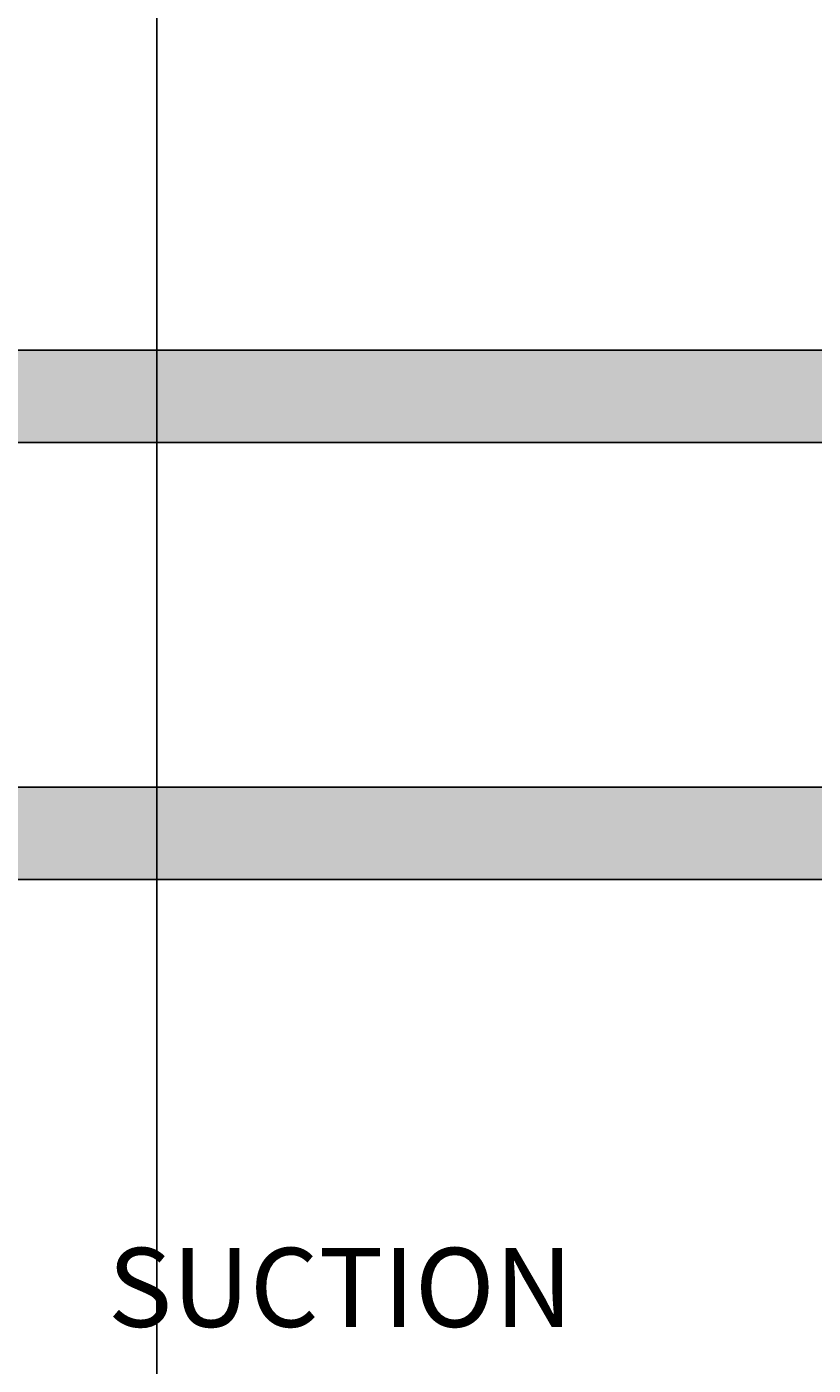
# Model space of a CAD drawing. Units: millimetres. Extents: x -11 to 280, y -4 to 208.
# Tile 5 of 55: x 61 to 91, y 36 to 87. Entities that reach past the tile are written whole.
import ezdxf

# ---------------------------------------------------------------- set-up
doc = ezdxf.new("R2010")
doc.units = ezdxf.units.MM
for name, color, linetype, lineweight in [('M-ANNO-TEXT', 7, 'Continuous', 18), ('M-DIMS', 2, 'Continuous', 18), ('M-HYDR-RETN', 7, 'Continuous', 25)]:
    doc.layers.add(name, color=color, linetype=linetype, lineweight=lineweight)
doc.layers.add('M-HYDR-RETN-PATT', color=114, linetype='Continuous', lineweight=13, true_color=0x139b48)
doc.styles.get("Standard").update_dxf_attribs({"font": 'arial.ttf'})
doc.dimstyles.get("Standard").update_dxf_attribs({"dimtxt": 0.18, "dimasz": 0.18, "dimexe": 0.18, "dimexo": 0.0625, "dimgap": 0.09, "dimtad": 0, "dimtih": 1, "dimtoh": 1, "dimdec": 4, "dimzin": 0, "dimdsep": 46, "dimtxsty": 'Standard', "dimcen": 0.09, "dimadec": 0, "dimazin": 0, "dimtfac": 1, "dimtdec": 4, "dimtofl": 0, "dimtmove": 0, "dimatfit": 3, "dimfxl": 1, "dimtolj": 1, "dimtzin": 0, "dimarcsym": 0})

# ---------------------------------------------------------------- blocks, each defined once
blk = doc.blocks.new('*D4')
at = {"layer": 'Defpoints', "color": 0, "transparency": 16777216}
for p in [(4.763, 84.426), (266.035, 51.733), (266.035, -3.415)]:
    blk.add_point(p, dxfattribs=at)
at = {"layer": 'M-DIMS', "color": 0, "lineweight": -2, "transparency": 16777216}
for p, q in [((4.763, 84.364), (4.763, -3.595)), ((266.035, 51.67), (266.035, -3.595)), ((4.943, -3.415), (134.934, -3.415)), ((265.855, -3.415), (135.864, -3.415))]:
    blk.add_line(p, q, dxfattribs=at)
at = {"layer": 'M-DIMS', "color": 0, "transparency": 16777216}
for points in [[(4.943, -3.385), (4.943, -3.445), (4.763, -3.415)], [(265.855, -3.385), (265.855, -3.445), (266.035, -3.415)]]:
    blk.add_solid(points, dxfattribs=at)
at = {"layer": 'M-DIMS', "color": 0, "transparency": 16777216, "insert": (135.399, -3.415), "char_height": 0.18, "attachment_point": 5}
blk.add_mtext('\\A1;261.27', dxfattribs=at)
blk = doc.blocks.new('*D5')
at = {"layer": 'Defpoints', "color": 0, "transparency": 16777216}
for p in [(24.759, 192.645), (-10.087, 11.435), (261.686, 11.435)]:
    blk.add_point(p, dxfattribs=at)
at = {"layer": 'M-DIMS', "color": 0, "lineweight": -2, "transparency": 16777216}
for p, q in [((24.696, 192.645), (-10.267, 192.645)), ((-10.087, 192.465), (-10.087, 102.222)), ((-10.087, 11.615), (-10.087, 101.858)), ((261.624, 11.435), (-10.267, 11.435))]:
    blk.add_line(p, q, dxfattribs=at)
at = {"layer": 'M-DIMS', "color": 0, "transparency": 16777216}
for points in [[(-10.117, 192.465), (-10.057, 192.465), (-10.087, 192.645)], [(-10.117, 11.615), (-10.057, 11.615), (-10.087, 11.435)]]:
    blk.add_solid(points, dxfattribs=at)
at = {"layer": 'M-DIMS', "color": 0, "transparency": 16777216, "insert": (-10.087, 102.04), "char_height": 0.18, "attachment_point": 5}
blk.add_mtext('\\A1;181.2', dxfattribs=at)
blk = doc.blocks.new('*D23')
at = {"layer": 'Defpoints', "color": 0, "transparency": 16777216}
for p in [(29.201, 153.977), (66.388, 153.977), (66.388, -3.415)]:
    blk.add_point(p, dxfattribs=at)
at = {"layer": 'M-DIMS', "color": 0, "lineweight": -2, "transparency": 16777216}
for p, q in [((29.201, 153.914), (29.201, -3.595)), ((66.388, 153.914), (66.388, -3.595)), ((29.381, -3.415), (47.331, -3.415)), ((66.208, -3.415), (48.258, -3.415))]:
    blk.add_line(p, q, dxfattribs=at)
at = {"layer": 'M-DIMS', "color": 0, "transparency": 16777216}
for points in [[(29.381, -3.385), (29.381, -3.445), (29.201, -3.415)], [(66.208, -3.385), (66.208, -3.445), (66.388, -3.415)]]:
    blk.add_solid(points, dxfattribs=at)
at = {"layer": 'M-DIMS', "color": 0, "transparency": 16777216, "insert": (47.795, -3.415), "char_height": 0.18, "attachment_point": 5}
blk.add_mtext('\\A1;37.186', dxfattribs=at)

msp = doc.modelspace()

# ---------------------------------------------------------------- hatches: boundary and pattern name
at = {"layer": 'M-HYDR-RETN-PATT'}
h = msp.add_hatch(color=256, dxfattribs=at)
h.set_gradient(color1=(19, 155, 72), color2=(19, 155, 72), tint=1)
h.paths.add_polyline_path([(17.9701, 159.0814), (29.2015, 159.0814), (29.2015, 162.5814), (14.4701, 162.5814), (14.4701, 98.0213), (17.9701, 98.0213)])
h.paths.add_polyline_path([(17.9701, 84.4261), (14.4701, 84.4261), (14.4701, 54.3099), (156.2446, 54.3099), (156.2446, 57.8099), (17.9701, 57.8099)])
h.paths.add_polyline_path([(120.5137, 74.3991), (17.9701, 74.3991), (17.9701, 70.8991), (120.5137, 70.8991)], flags=17)
h.paths.add_polyline_path([(184.7092, 75.04, 0.4142136), (179.7092, 80.04), (156.2446, 80.04), (156.2446, 57.8099), (156.2446, 54.3099), (156.2446, 43.5991), (159.7446, 43.5991), (159.7446, 57.8099), (159.7446, 76.54), (176.2092, 76.54, -0.4142136), (181.2092, 71.54), (181.2092, 57.8099), (159.7446, 57.8099), (159.7446, 54.3099), (184.7092, 54.3099)])

# ---------------------------------------------------------------- linework, layer by layer
at = {"layer": 'M-HYDR-RETN'}
for points in [[(14.4701, 84.4261), (14.4701, 54.3099), (156.2446, 54.3099)], [(17.9701, 84.4261), (17.9701, 57.8099), (156.2446, 57.8099)], [(17.9701, 74.3991), (120.5137, 74.3991)], [(17.9701, 70.8991), (120.5137, 70.8991)]]:
    msp.add_lwpolyline(points, dxfattribs=at)

# ---------------------------------------------------------------- texts
at = {"layer": 'M-ANNO-TEXT', "insert": (64.5255, 40.3159), "char_height": 3, "attachment_point": 1}
msp.add_mtext_dynamic_manual_height_columns('SUCTION', width=31.695986, gutter_width=12.5, heights=[0], dxfattribs=at)

# ---------------------------------------------------------------- dimensions: what is measured, and where the dimension line sits
at = {"layer": 'M-DIMS'}
dim = msp.add_linear_dim(base=(-10.0865, 11.4346), p1=(24.7588, 192.645), p2=(261.6863, 11.4346), angle=90, dimstyle='Standard', override={"dimdec": 1, "dimlfac": 1, "dimrnd": 0, "dimzin": 0, "dimdsep": 46, "dimlunit": 2}, dxfattribs=at)
dim.commit()
dim.dimension.update_dxf_attribs({"geometry": '*D5', "text_midpoint": (-10.0865, 102.0398)})
for base, p1, p2, override, picture, middle in [((66.3875, -3.4154), (29.2015, 153.9768), (66.3875, 153.9768), {"dimdec": 3, "dimlfac": 1, "dimrnd": 0, "dimzin": 0, "dimdsep": 46, "dimlunit": 2}, '*D23', (47.7945, -3.4154)), ((266.0352, -3.4154), (4.7635, 84.4261), (266.0352, 51.7328), {"dimdec": 2, "dimlfac": 1, "dimrnd": 0, "dimzin": 0, "dimdsep": 46, "dimlunit": 2}, '*D4', (135.3993, -3.4154))]:
    dim = msp.add_linear_dim(base=base, p1=p1, p2=p2, dimstyle='Standard', override=override, dxfattribs=at)
    dim.commit()
    dim.dimension.update_dxf_attribs({"geometry": picture, "text_midpoint": middle})

doc.saveas('drawing.dxf')
